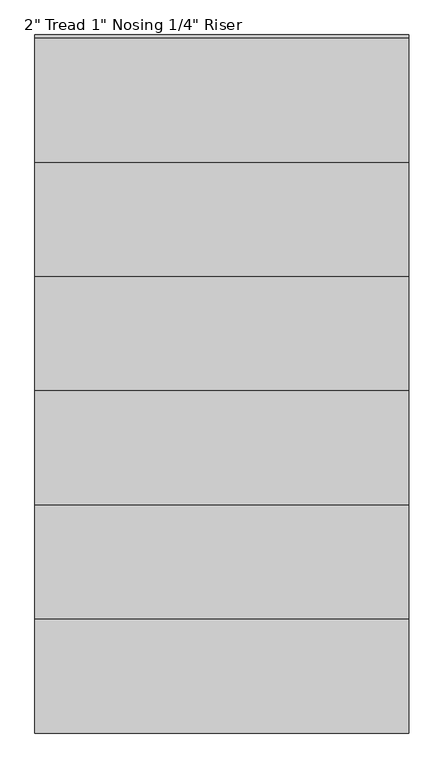
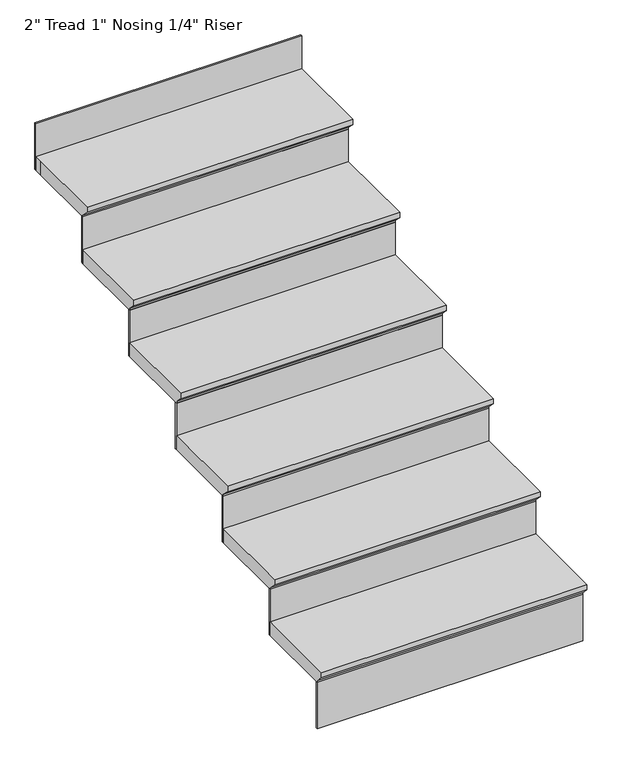
"""IFC4 building model written with IfcOpenShell, lengths in millimetres: stair flight geometry."""

from ifc_helpers import new_model, si_unit, origin, place, context, project, spatial, faceted_brep, source, transform, mapped, element, save


def stair_flight_2e9a7ce1(model_context):
    return source(origin(), model_context, "Body", "Brep", [
        faceted_brep([(4429.2597674, -1341.8241735, 1166.2833333), (4429.2597674, -1341.8241735, 1185.3333333), (3514.8597674, -1341.8241735, 1185.3333333), (3514.8597674, -1341.8241735, 1166.2833333), (4429.2597674, -1316.4241735, 1140.8833333), (3514.8597674, -1316.4241735, 1140.8833333), (4429.2597674, -1037.0241735, 1185.3333333), (3514.8597674, -1037.0241735, 1185.3333333), (3514.8597674, -1316.4241735, 1134.5333333), (3514.8597674, -1037.0241735, 1134.5333333), (4429.2597674, -1037.0241735, 1134.5333333), (4429.2597674, -1316.4241735, 1134.5333333)], [[[0, 1, 2, 3]], [[4, 0, 3, 5]], [[2, 1, 6, 7]], [[8, 9, 10, 11]], [[2, 7, 9, 8, 5, 3]], [[8, 11, 4, 5]], [[6, 1, 0, 4, 11, 10]], [[7, 6, 10, 9]]]),
        faceted_brep([(4429.2597674, -1316.4241735, 1134.5333333), (4429.2597674, -1316.4241735, 965.2), (4429.2597674, -1310.0741735, 965.2), (4429.2597674, -1310.0741735, 1134.5333333), (3514.8597674, -1316.4241735, 1134.5333333), (3514.8597674, -1310.0741735, 1134.5333333), (3514.8597674, -1310.0741735, 965.2), (3514.8597674, -1316.4241735, 965.2)], [[[0, 1, 2, 3]], [[4, 5, 6, 7]], [[1, 0, 4, 7]], [[2, 1, 7, 6]], [[3, 2, 6, 5]], [[0, 3, 5, 4]]]),
        faceted_brep([(4429.2597674, -1037.0241735, 1303.8666667), (4429.2597674, -1037.0241735, 1134.5333333), (4429.2597674, -1030.6741735, 1134.5333333), (4429.2597674, -1030.6741735, 1303.8666667), (3514.8597674, -1037.0241735, 1303.8666667), (3514.8597674, -1030.6741735, 1303.8666667), (3514.8597674, -1030.6741735, 1134.5333333), (3514.8597674, -1037.0241735, 1134.5333333)], [[[0, 1, 2, 3]], [[4, 5, 6, 7]], [[1, 0, 4, 7]], [[2, 1, 7, 6]], [[3, 2, 6, 5]], [[0, 3, 5, 4]]]),
        faceted_brep([(3514.8597674, -1062.4241735, 1354.6666667), (4429.2597674, -1062.4241735, 1354.6666667), (4429.2597674, -757.6241735, 1354.6666667), (3514.8597674, -757.6241735, 1354.6666667), (3514.8597674, -1037.0241735, 1303.8666667), (3514.8597674, -757.6241735, 1303.8666667), (4429.2597674, -757.6241735, 1303.8666667), (4429.2597674, -1037.0241735, 1303.8666667), (3514.8597674, -1037.0241735, 1310.2166667), (3514.8597674, -1062.4241735, 1335.6166667), (4429.2597674, -1037.0241735, 1310.2166667), (4429.2597674, -1062.4241735, 1335.6166667)], [[[0, 1, 2, 3]], [[4, 5, 6, 7]], [[0, 3, 5, 4, 8, 9]], [[4, 7, 10, 8]], [[2, 1, 11, 10, 7, 6]], [[3, 2, 6, 5]], [[11, 1, 0, 9]], [[10, 11, 9, 8]]]),
        faceted_brep([(4429.2597674, -757.6241735, 1473.2), (4429.2597674, -757.6241735, 1303.8666667), (4429.2597674, -751.2741735, 1303.8666667), (4429.2597674, -751.2741735, 1473.2), (3514.8597674, -757.6241735, 1473.2), (3514.8597674, -751.2741735, 1473.2), (3514.8597674, -751.2741735, 1303.8666667), (3514.8597674, -757.6241735, 1303.8666667)], [[[0, 1, 2, 3]], [[4, 5, 6, 7]], [[1, 0, 4, 7]], [[2, 1, 7, 6]], [[3, 2, 6, 5]], [[0, 3, 5, 4]]]),
        faceted_brep([(3514.8597674, -783.0241735, 1524.0), (4429.2597674, -783.0241735, 1524.0), (4429.2597674, -478.2241735, 1524.0), (3514.8597674, -478.2241735, 1524.0), (3514.8597674, -757.6241735, 1473.2), (3514.8597674, -478.2241735, 1473.2), (4429.2597674, -478.2241735, 1473.2), (4429.2597674, -757.6241735, 1473.2), (3514.8597674, -757.6241735, 1479.55), (3514.8597674, -783.0241735, 1504.95), (4429.2597674, -757.6241735, 1479.55), (4429.2597674, -783.0241735, 1504.95)], [[[0, 1, 2, 3]], [[4, 5, 6, 7]], [[0, 3, 5, 4, 8, 9]], [[4, 7, 10, 8]], [[2, 1, 11, 10, 7, 6]], [[3, 2, 6, 5]], [[11, 1, 0, 9]], [[10, 11, 9, 8]]]),
        faceted_brep([(4429.2597674, -478.2241735, 1642.5333333), (4429.2597674, -478.2241735, 1473.2), (4429.2597674, -471.8741735, 1473.2), (4429.2597674, -471.8741735, 1642.5333333), (3514.8597674, -478.2241735, 1642.5333333), (3514.8597674, -471.8741735, 1642.5333333), (3514.8597674, -471.8741735, 1473.2), (3514.8597674, -478.2241735, 1473.2)], [[[0, 1, 2, 3]], [[4, 5, 6, 7]], [[1, 0, 4, 7]], [[2, 1, 7, 6]], [[3, 2, 6, 5]], [[0, 3, 5, 4]]]),
        faceted_brep([(3514.8597674, -503.6241735, 1693.3333333), (4429.2597674, -503.6241735, 1693.3333333), (4429.2597674, -198.8241735, 1693.3333333), (3514.8597674, -198.8241735, 1693.3333333), (3514.8597674, -478.2241735, 1642.5333333), (3514.8597674, -198.8241735, 1642.5333333), (4429.2597674, -198.8241735, 1642.5333333), (4429.2597674, -478.2241735, 1642.5333333), (3514.8597674, -478.2241735, 1648.8833333), (3514.8597674, -503.6241735, 1674.2833333), (4429.2597674, -478.2241735, 1648.8833333), (4429.2597674, -503.6241735, 1674.2833333)], [[[0, 1, 2, 3]], [[4, 5, 6, 7]], [[0, 3, 5, 4, 8, 9]], [[4, 7, 10, 8]], [[2, 1, 11, 10, 7, 6]], [[3, 2, 6, 5]], [[11, 1, 0, 9]], [[10, 11, 9, 8]]]),
        faceted_brep([(4429.2597674, -198.8241735, 1811.8666667), (4429.2597674, -198.8241735, 1642.5333333), (4429.2597674, -192.4741735, 1642.5333333), (4429.2597674, -192.4741735, 1811.8666667), (3514.8597674, -198.8241735, 1811.8666667), (3514.8597674, -192.4741735, 1811.8666667), (3514.8597674, -192.4741735, 1642.5333333), (3514.8597674, -198.8241735, 1642.5333333)], [[[0, 1, 2, 3]], [[4, 5, 6, 7]], [[1, 0, 4, 7]], [[2, 1, 7, 6]], [[3, 2, 6, 5]], [[0, 3, 5, 4]]]),
        faceted_brep([(3514.8597674, -224.2241735, 1862.6666667), (4429.2597674, -224.2241735, 1862.6666667), (4429.2597674, 80.5758265, 1862.6666667), (3514.8597674, 80.5758265, 1862.6666667), (3514.8597674, -198.8241735, 1811.8666667), (3514.8597674, 80.5758265, 1811.8666667), (4429.2597674, 80.5758265, 1811.8666667), (4429.2597674, -198.8241735, 1811.8666667), (3514.8597674, -198.8241735, 1818.2166667), (3514.8597674, -224.2241735, 1843.6166667), (4429.2597674, -198.8241735, 1818.2166667), (4429.2597674, -224.2241735, 1843.6166667)], [[[0, 1, 2, 3]], [[4, 5, 6, 7]], [[0, 3, 5, 4, 8, 9]], [[4, 7, 10, 8]], [[2, 1, 11, 10, 7, 6]], [[3, 2, 6, 5]], [[11, 1, 0, 9]], [[10, 11, 9, 8]]]),
        faceted_brep([(4429.2597674, 359.9758265, 2150.5333333), (4429.2597674, 359.9758265, 1981.2), (4429.2597674, 366.3258265, 1981.2), (4429.2597674, 366.3258265, 2150.5333333), (3514.8597674, 359.9758265, 2150.5333333), (3514.8597674, 366.3258265, 2150.5333333), (3514.8597674, 366.3258265, 1981.2), (3514.8597674, 359.9758265, 1981.2)], [[[0, 1, 2, 3]], [[4, 5, 6, 7]], [[1, 0, 4, 7]], [[2, 1, 7, 6]], [[3, 2, 6, 5]], [[0, 3, 5, 4]]]),
        faceted_brep([(4429.2597674, 80.5758265, 1981.2), (4429.2597674, 80.5758265, 1811.8666667), (4429.2597674, 86.9258265, 1811.8666667), (4429.2597674, 86.9258265, 1981.2), (3514.8597674, 80.5758265, 1981.2), (3514.8597674, 86.9258265, 1981.2), (3514.8597674, 86.9258265, 1811.8666667), (3514.8597674, 80.5758265, 1811.8666667)], [[[0, 1, 2, 3]], [[4, 5, 6, 7]], [[1, 0, 4, 7]], [[2, 1, 7, 6]], [[3, 2, 6, 5]], [[0, 3, 5, 4]]]),
        faceted_brep([(3514.8597674, 359.9758265, 2032.0), (3514.8597674, 334.5758265, 2032.0), (3514.8597674, 55.1758265, 2032.0), (4429.2597674, 55.1758265, 2032.0), (4429.2597674, 334.5758265, 2032.0), (4429.2597674, 359.9758265, 2032.0), (3514.8597674, 334.5758265, 1981.2), (3514.8597674, 359.9758265, 1981.2), (4429.2597674, 359.9758265, 1981.2), (4429.2597674, 334.5758265, 1981.2), (4429.2597674, 80.5758265, 1981.2), (3514.8597674, 80.5758265, 1981.2), (3514.8597674, 80.5758265, 1987.55), (3514.8597674, 55.1758265, 2012.95), (4429.2597674, 80.5758265, 1987.55), (4429.2597674, 55.1758265, 2012.95)], [[[0, 1, 2, 3, 4, 5]], [[6, 7, 8, 9, 10, 11]], [[1, 0, 7, 6]], [[2, 1, 6, 11, 12, 13]], [[11, 10, 14, 12]], [[4, 3, 15, 14, 10, 9]], [[5, 4, 9, 8]], [[0, 5, 8, 7]], [[15, 3, 2, 13]], [[14, 15, 13, 12]]]),
    ])


if __name__ == "__main__":
    model = new_model("IFC4")
    model_context = context("Model", 3, world=origin())
    ifc_project = project(units=[si_unit("LENGTHUNIT", "METRE", prefix="MILLI")], contexts=[model_context])
    site = spatial("IfcSite", under=ifc_project)
    building = spatial("IfcBuilding", under=site)
    placement = place(None, origin())
    stair_flight_shape = stair_flight_2e9a7ce1(model_context)
    element("IfcStairFlight", 1, ObjectType="2\" Tread 1\" Nosing 1/4\" Riser", at=placement, inside=building, context=model_context, shape_type="MappedRepresentation", body=[
        mapped(stair_flight_shape, transform((0.0, 0.0, 0.0), x_axis=(1.0, 0.0, 0.0), y_axis=(0.0, 1.0, 0.0), z_axis=(0.0, 0.0, 1.0))),
    ])
    save(model, "model.ifc")
